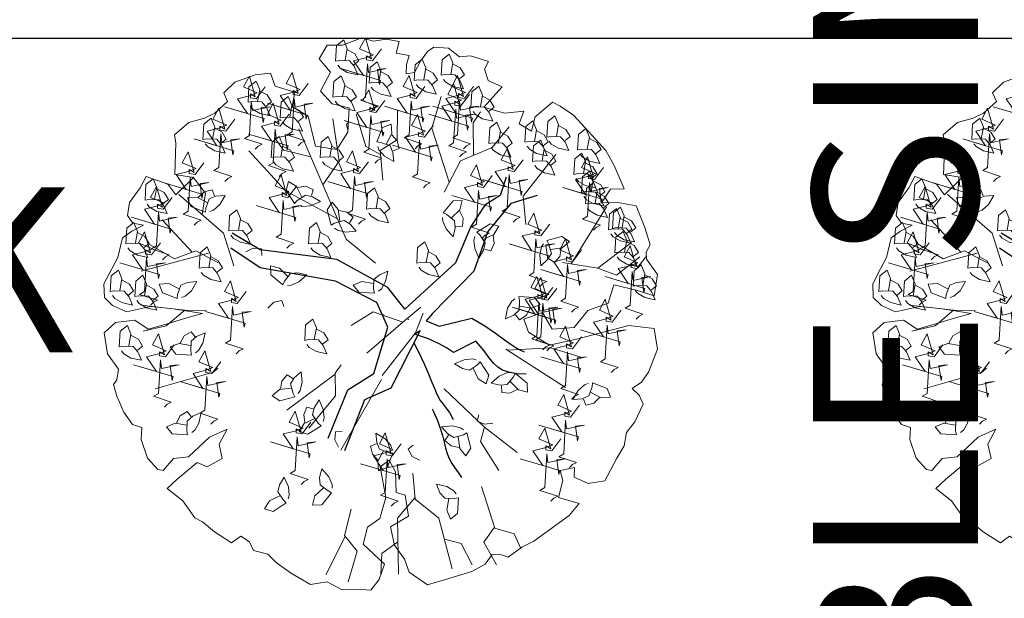
# Model space of a CAD drawing. Units: inches. Extents: x 2831 to 4250, y 1103 to 1797.
# Tile 10 of 15: x 3676 to 3730, y 1690 to 1722. Entities that reach past the tile are written whole.
import ezdxf

# ---------------------------------------------------------------- set-up
doc = ezdxf.new("R2010")
doc.units = ezdxf.units.IN
for name, color, linetype, lineweight in [('A-ANNO-DIMS', 2, 'Continuous', 18), ('A-ANNO-TEXT', 7, 'Continuous', 18), ('A-WALL-PATT', 252, 'Continuous', 13), ('ARBOL', 30, 'Continuous', 13), ('C-PROP', 7, 'Continuous', 25)]:
    doc.layers.add(name, color=color, linetype=linetype, lineweight=lineweight)
doc.layers.add('TALLO', color=36, linetype='Continuous')
doc.styles.get("Standard").update_dxf_attribs({"font": 'arial.ttf'})
doc.dimstyles.new('ISO-25', dxfattribs={"dimtxt": 9, "dimasz": 2.5, "dimexe": 1.25, "dimexo": 0.625, "dimtad": 1, "dimdec": 1, "dimlunit": 3, "dimtxsty": 'Standard', "dimcen": 2.5, "dimadec": 0, "dimazin": 0, "dimtfac": 1, "dimtdec": 1, "dimtmove": 0, "dimatfit": 3, "dimfxl": 1, "dimarcsym": 0})

# ---------------------------------------------------------------- blocks, each defined once
blk = doc.blocks.new('fresno')
at = {"layer": 'ARBOL'}
for p, q in [((2.96, 0.991), (3.575, 1.984)), ((-3.638, 1.194), (-4.164, 1.76)), ((-1.151, -0.932), (-1.99, -1.556)), ((-0.974, -3.757), (-1.31, -4.423))]:
    blk.add_line(p, q, dxfattribs=at)
blk.add_lwpolyline([(0.823, 4.745), (0.566, 4.764), (0.459, 4.687), (0.336, 4.518), (0.233, 4.322), (0.087, 4.298), (0.091, 4.464), (0.14, 4.621), (-0.09, 4.659), (-0.033, 4.863), (-0.264, 4.901), (-0.483, 4.866), (-0.686, 4.924), (-1.021, 4.801), (-1.288, 4.8), (-1.431, 4.563), (-1.234, 4.327), (-1.406, 4), (-1.205, 3.778), (-0.909, 3.705), (-0.931, 3.283), (-1.122, 2.983), (-1.491, 3.043), (-1.619, 3.562), (-1.9, 3.727), (-1.851, 3.982), (-2.197, 4.084), (-2.278, 4.31), (-2.543, 4.283), (-2.896, 4.152), (-3.091, 3.971), (-3.022, 3.817), (-3.244, 3.617), (-3.424, 3.528), (-3.697, 3.455), (-3.946, 3.236), (-3.922, 3.09), (-3.94, 2.548), (-3.617, 2.495), (-3.927, 2.19), (-4.062, 2.379), (-4.443, 2.512), (-4.546, 2.316), (-4.73, 2.062), (-4.767, 1.832), (-4.671, 1.698), (-4.486, 1.667), (-4.693, 1.559), (-4.854, 1.444), (-4.934, 1.102), (-5.037, 0.905), (-5.175, 0.644), (-5.166, 0.406), (-5.024, 0.264), (-4.781, 0.153), (-4.363, 0.249), (-4.014, 0.215), (-3.783, 0.177), (-3.46, 0.124), (-3.733, 0.051), (-4.132, -0.073), (-4.404, -0.146), (-4.639, 0.011), (-4.977, -0.028), (-5.172, -0.209), (-5.113, -0.574), (-4.921, -0.843), (-4.951, -1.027), (-5.012, -1.112), (-4.95, -1.311), (-4.83, -1.592), (-4.676, -1.807), (-4.518, -1.856), (-4.529, -2.068), (-4.417, -2.394), (-4.236, -2.59), (-4.143, -2.605), (-3.967, -2.397), (-3.703, -2.37), (-3.339, -2.027), (-3.032, -1.889), (-3.169, -2.15), (-3.115, -2.396), (-3.376, -2.542), (-3.552, -2.466), (-3.909, -2.762), (-4.077, -2.924), (-3.804, -3.135), (-3.592, -3.43), (-3.461, -3.499), (-3.253, -3.676), (-2.953, -3.867), (-2.792, -3.752), (-2.642, -3.848), (-2.572, -4.001), (-2.323, -4.066), (-2.18, -4.208), (-1.926, -4.392), (-1.58, -4.591), (-1.288, -4.545), (-1.027, -4.683), (-0.788, -4.675), (-0.531, -4.693), (-0.382, -4.505), (-0.29, -4.236), (-0.66, -3.891), (-0.588, -3.595), (-0.374, -3.441), (-0.267, -3.079), (-0.368, -2.541), (-0.208, -2.426), (-0.099, -2.633), (-0.087, -2.991), (0.071, -3.04), (0.129, -3.405), (-0.185, -3.59), (-0.119, -3.909), (0.055, -4.151), (0.136, -4.377), (0.456, -4.596), (0.828, -4.491), (1.227, -4.368), (1.461, -4.241), (1.583, -4.071), (1.748, -4.075), (1.86, -4.117), (2.101, -3.944), (2.308, -3.836), (2.925, -3.393), (3.101, -3.185), (2.74, -3.078), (2.812, -2.782), (2.769, -2.61), (3.015, -2.555), (3.012, -2.721), (3.254, -2.832), (3.546, -2.785), (3.752, -2.393), (3.882, -2.177), (3.92, -1.947), (4.069, -1.758), (4.214, -1.451), (4.144, -1.297), (4.021, -1.182), (4.182, -1.067), (4.304, -0.897), (4.464, -0.497), (4.429, -0.279), (4.406, -0.133), (3.964, -0.083), (3.074, -0.315), (2.582, -0.424), (2.217, -0.197), (2.136, 0.029), (2.462, 0.141), (2.628, -0.147), (3.012, -0.116), (3.249, 0.177), (3.602, 0.308), (3.701, 0.623), (4.089, 0.535), (4.404, 0.436), (4.464, 0.805), (4.272, 1.074), (4.267, 1.193), (4.336, 1.324), (4.243, 1.623), (4.092, 2.003), (3.769, 2.057), (3.485, 2.056), (3.642, 2.291), (3.88, 2.299), (3.71, 2.706), (3.563, 2.967), (3.201, 3.358), (3.001, 3.581), (2.766, 3.738), (2.635, 3.807), (2.332, 3.549), (2.268, 3.299), (2.052, 3.429), (2.136, 3.652), (1.798, 3.613), (1.437, 3.72), (1.755, 4.071), (1.513, 4.182), (1.451, 4.381), (1.519, 4.512), (1.204, 4.611), (1.012, 4.596)], close=True, dxfattribs=at)
for points in [[(-1.104, 4.45), (-1.063, 4.399), (-0.939, 4.325), (-0.757, 4.285), (-0.82, 4.431), (-0.903, 4.527), (-1.075, 4.533), (-1.143, 4.521), (-1.126, 4.792), (-1.002, 4.891), (-0.939, 4.738), (-0.975, 4.535)], [(-0.346, 4.735), (-0.501, 4.528), (-0.605, 4.545), (-0.605, 4.614), (-0.519, 4.563), (-0.622, 4.925), (-0.726, 4.735), (-0.484, 4.632), (-0.622, 4.58), (-0.829, 4.528), (-0.657, 4.27), (-1.053, 4.39), (-0.363, 4.183), (-0.381, 4.114), (-0.415, 4.373), (-0.26, 4.39), (-0.57, 4.321), (-0.588, 4.476), (-0.622, 3.89), (-0.708, 3.839), (-0.398, 3.735), (-0.467, 3.701), (-0.519, 3.649)], [(-0.935, 4.717), (-0.809, 4.65), (-0.736, 4.529), (-0.824, 4.459)], [(0.734, 4.203), (0.775, 4.152), (0.9, 4.078), (1.082, 4.038), (1.018, 4.185), (0.936, 4.281), (0.763, 4.287), (0.696, 4.274), (0.712, 4.546), (0.837, 4.645), (0.899, 4.491), (0.863, 4.289)], [(-0.521, 4.069), (-0.48, 4.018), (-0.356, 3.944), (-0.174, 3.904), (-0.237, 4.051), (-0.32, 4.146), (-0.492, 4.152), (-0.56, 4.14), (-0.543, 4.411), (-0.419, 4.511), (-0.356, 4.357), (-0.392, 4.154)], [(0.263, 4.114), (0.304, 4.063), (0.429, 3.989), (0.611, 3.948), (0.547, 4.095), (0.465, 4.191), (0.293, 4.197), (0.225, 4.185), (0.242, 4.456), (0.366, 4.555), (0.428, 4.402), (0.393, 4.199)], [(0.904, 4.471), (1.029, 4.404), (1.102, 4.282), (1.015, 4.212)], [(-1.623, 4.132), (-1.778, 3.925), (-1.882, 3.942), (-1.882, 4.011), (-1.795, 3.959), (-1.899, 4.321), (-2.002, 4.132), (-1.761, 4.028), (-1.899, 3.977), (-2.106, 3.925), (-1.933, 3.666), (-2.33, 3.787), (-1.64, 3.58), (-1.657, 3.511), (-1.692, 3.77), (-1.537, 3.787), (-1.847, 3.718), (-1.864, 3.873), (-1.899, 3.287), (-1.985, 3.235), (-1.675, 3.132), (-1.744, 3.097), (-1.795, 3.046)], [(-0.352, 4.337), (-0.226, 4.269), (-0.153, 4.148), (-0.241, 4.078)], [(0.433, 4.381), (0.558, 4.314), (0.631, 4.193), (0.544, 4.122)], [(-2.368, 4.073), (-2.523, 3.866), (-2.627, 3.883), (-2.627, 3.952), (-2.541, 3.9), (-2.644, 4.262), (-2.748, 4.073), (-2.506, 3.969), (-2.644, 3.918), (-2.851, 3.866), (-2.679, 3.607), (-3.075, 3.728), (-2.385, 3.521), (-2.403, 3.452), (-2.437, 3.711), (-2.282, 3.728), (-2.592, 3.659), (-2.61, 3.814), (-2.644, 3.228), (-2.73, 3.176), (-2.42, 3.073), (-2.489, 3.038), (-2.541, 2.987)], [(-2.629, 3.733), (-2.588, 3.682), (-2.463, 3.608), (-2.281, 3.568), (-2.345, 3.715), (-2.427, 3.81), (-2.6, 3.816), (-2.667, 3.804), (-2.651, 4.075), (-2.526, 4.175), (-2.464, 4.021), (-2.5, 3.818)], [(-1.149, 3.822), (-1.108, 3.771), (-0.983, 3.697), (-0.802, 3.657), (-0.865, 3.804), (-0.948, 3.9), (-1.12, 3.906), (-1.188, 3.893), (-1.171, 4.165), (-1.047, 4.264), (-0.984, 4.111), (-1.02, 3.908)], [(0.413, 4.08), (0.258, 3.873), (0.154, 3.89), (0.154, 3.959), (0.241, 3.908), (0.137, 4.27), (0.034, 4.08), (0.275, 3.977), (0.137, 3.925), (-0.07, 3.873), (0.103, 3.614), (-0.294, 3.735), (0.396, 3.528), (0.379, 3.459), (0.344, 3.718), (0.499, 3.735), (0.189, 3.666), (0.172, 3.821), (0.137, 3.235), (0.051, 3.183), (0.361, 3.08), (0.292, 3.046), (0.241, 2.994)], [(1.189, 3.942), (1.034, 3.735), (0.931, 3.752), (0.931, 3.821), (1.017, 3.77), (0.913, 4.132), (0.81, 3.942), (1.051, 3.839), (0.913, 3.787), (0.706, 3.735), (0.879, 3.477), (0.482, 3.597), (1.172, 3.39), (1.155, 3.321), (1.12, 3.58), (1.276, 3.597), (0.965, 3.528), (0.948, 3.683), (0.913, 3.097), (0.827, 3.046), (1.138, 2.942), (1.069, 2.908), (1.017, 2.856)], [(1.259, 4.08), (1.103, 3.873), (1, 3.89), (1, 3.959), (1.086, 3.908), (0.982, 4.27), (0.879, 4.08), (1.12, 3.977), (0.982, 3.925), (0.775, 3.873), (0.948, 3.614), (0.551, 3.735), (1.241, 3.528), (1.224, 3.459), (1.189, 3.718), (1.345, 3.735), (1.034, 3.666), (1.017, 3.821), (0.982, 3.235), (0.896, 3.183), (1.207, 3.08), (1.138, 3.046), (1.086, 2.994)], [(-2.459, 4), (-2.334, 3.933), (-2.261, 3.812), (-2.348, 3.742)], [(-0.287, 3.833), (-0.442, 3.626), (-0.546, 3.643), (-0.546, 3.712), (-0.46, 3.661), (-0.563, 4.023), (-0.667, 3.833), (-0.425, 3.73), (-0.563, 3.678), (-0.77, 3.626), (-0.598, 3.367), (-0.995, 3.488), (-0.304, 3.281), (-0.322, 3.212), (-0.356, 3.471), (-0.201, 3.488), (-0.511, 3.419), (-0.529, 3.574), (-0.563, 2.988), (-0.649, 2.936), (-0.339, 2.833), (-0.408, 2.799), (-0.46, 2.747)], [(-0.98, 4.09), (-0.854, 4.023), (-0.781, 3.901), (-0.869, 3.831)], [(1.25, 3.643), (1.291, 3.592), (1.416, 3.518), (1.597, 3.478), (1.534, 3.625), (1.451, 3.721), (1.279, 3.727), (1.211, 3.714), (1.228, 3.985), (1.352, 4.085), (1.415, 3.931), (1.379, 3.729)], [(-1.951, 3.597), (-2.106, 3.39), (-2.209, 3.408), (-2.209, 3.477), (-2.123, 3.425), (-2.227, 3.787), (-2.33, 3.597), (-2.089, 3.494), (-2.227, 3.442), (-2.434, 3.39), (-2.261, 3.132), (-2.658, 3.252), (-1.968, 3.046), (-1.985, 2.977), (-2.02, 3.235), (-1.864, 3.252), (-2.175, 3.183), (-2.192, 3.339), (-2.227, 2.752), (-2.313, 2.701), (-2.002, 2.597), (-2.071, 2.563), (-2.123, 2.511)], [(-2.068, 3.464), (-2.027, 3.413), (-1.903, 3.339), (-1.721, 3.299), (-1.784, 3.446), (-1.867, 3.542), (-2.039, 3.547), (-2.107, 3.535), (-2.09, 3.806), (-1.966, 3.906), (-1.903, 3.752), (-1.939, 3.55)], [(0.837, 2.414), (0.533, 3.352), (0.697, 3.906)], [(1.419, 3.911), (1.545, 3.844), (1.618, 3.722), (1.53, 3.652)], [(-2.898, 3.511), (-3.053, 3.304), (-3.157, 3.321), (-3.157, 3.39), (-3.071, 3.339), (-3.174, 3.701), (-3.278, 3.511), (-3.036, 3.408), (-3.174, 3.356), (-3.381, 3.304), (-3.209, 3.046), (-3.605, 3.166), (-2.915, 2.959), (-2.932, 2.89), (-2.967, 3.149), (-2.812, 3.166), (-3.122, 3.097), (-3.14, 3.253), (-3.174, 2.666), (-3.26, 2.615), (-2.95, 2.511), (-3.019, 2.477), (-3.071, 2.425)], [(-1.899, 3.732), (-1.773, 3.664), (-1.7, 3.543), (-1.788, 3.473)], [(-0.063, 3.671), (-0.069, 3.151), (-0.364, 2.965), (-0.319, 2.449)], [(1.259, 2.882), (1.254, 3.446), (1.381, 3.636)], [(-3.413, 3.083), (-3.373, 3.032), (-3.248, 2.958), (-3.066, 2.918), (-3.129, 3.065), (-3.212, 3.161), (-3.384, 3.167), (-3.452, 3.154), (-3.435, 3.425), (-3.311, 3.525), (-3.248, 3.371), (-3.284, 3.169)], [(-1.367, 2.367), (-1.081, 2.78), (-1.193, 3.514)], [(-0.923, 3.449), (-0.951, 3.425), (-0.93, 3.313)], [(-0.358, 2.895), (-0.615, 3.037), (-0.783, 3.596)], [(0.558, 3.402), (0.403, 3.195), (0.299, 3.212), (0.299, 3.281), (0.386, 3.23), (0.282, 3.592), (0.179, 3.402), (0.42, 3.299), (0.282, 3.247), (0.075, 3.195), (0.248, 2.936), (-0.149, 3.057), (0.541, 2.85), (0.524, 2.781), (0.489, 3.04), (0.644, 3.057), (0.334, 2.988), (0.317, 3.143), (0.282, 2.557), (0.196, 2.505), (0.506, 2.402), (0.437, 2.368), (0.386, 2.316)], [(1.564, 3.016), (1.605, 2.965), (1.729, 2.891), (1.911, 2.851), (1.848, 2.998), (1.765, 3.094), (1.593, 3.099), (1.525, 3.087), (1.542, 3.358), (1.666, 3.458), (1.729, 3.304), (1.693, 3.102)], [(2.191, 3.038), (2.232, 2.987), (2.357, 2.913), (2.539, 2.873), (2.475, 3.02), (2.393, 3.116), (2.221, 3.122), (2.153, 3.109), (2.17, 3.381), (2.294, 3.48), (2.356, 3.326), (2.321, 3.124)], [(2.573, 3.128), (2.613, 3.077), (2.738, 3.003), (2.92, 2.963), (2.857, 3.11), (2.774, 3.205), (2.602, 3.211), (2.534, 3.199), (2.551, 3.47), (2.675, 3.57), (2.738, 3.416), (2.702, 3.214)], [(-3.244, 3.351), (-3.118, 3.284), (-3.045, 3.162), (-3.133, 3.092)], [(-0.448, 1), (-0.961, 1.419), (-1.784, 3.341)], [(-0.41, 3.035), (-0.387, 2.974), (-0.291, 2.865), (-0.131, 2.771), (-0.146, 2.93), (-0.195, 3.047), (-0.357, 3.106), (-0.425, 3.115), (-0.325, 3.368), (-0.176, 3.424), (-0.164, 3.258), (-0.261, 3.077)], [(0.746, 2.242), (1.034, 2.786), (1.584, 3.019), (1.879, 3.374)], [(1.733, 3.284), (1.859, 3.216), (1.932, 3.095), (1.844, 3.025)], [(2.361, 3.306), (2.486, 3.239), (2.559, 3.117), (2.472, 3.047)], [(2.742, 3.396), (2.868, 3.328), (2.941, 3.207), (2.853, 3.137)], [(3.111, 2.904), (3.152, 2.853), (3.276, 2.779), (3.458, 2.739), (3.395, 2.886), (3.312, 2.981), (3.14, 2.987), (3.072, 2.975), (3.089, 3.246), (3.213, 3.346), (3.276, 3.192), (3.24, 2.99)], [(-2.225, 2.77), (-2.184, 2.718), (-2.06, 2.645), (-1.878, 2.604), (-1.941, 2.751), (-2.024, 2.847), (-2.196, 2.853), (-2.264, 2.84), (-2.247, 3.112), (-2.123, 3.211), (-2.06, 3.058), (-2.096, 2.855)], [(-1.575, 2.854), (-2.052, 2.969), (-2.2, 3.178)], [(-1.373, 2.77), (-1.332, 2.718), (-1.208, 2.645), (-1.026, 2.604), (-1.089, 2.751), (-1.172, 2.847), (-1.344, 2.853), (-1.412, 2.84), (-1.395, 3.112), (-1.271, 3.211), (-1.208, 3.058), (-1.244, 2.855)], [(-0.166, 3.238), (-0.068, 3.135), (-0.036, 2.997), (-0.141, 2.957)], [(2.326, 2.702), (2.367, 2.651), (2.492, 2.577), (2.673, 2.537), (2.61, 2.684), (2.527, 2.78), (2.355, 2.786), (2.287, 2.773), (2.304, 3.045), (2.428, 3.144), (2.491, 2.99), (2.455, 2.788)], [(3.28, 3.172), (3.406, 3.104), (3.479, 2.983), (3.391, 2.913)], [(-3.434, 2.752), (-3.59, 2.546), (-3.693, 2.563), (-3.693, 2.632), (-3.607, 2.58), (-3.71, 2.942), (-3.814, 2.752), (-3.572, 2.649), (-3.71, 2.597), (-3.917, 2.546), (-3.745, 2.287), (-4.142, 2.408), (-3.452, 2.201), (-3.469, 2.132), (-3.503, 2.39), (-3.348, 2.408), (-3.659, 2.339), (-3.676, 2.494), (-3.71, 1.908), (-3.797, 1.856), (-3.486, 1.753), (-3.555, 1.718), (-3.607, 1.666)], [(-1.112, 1.773), (-2.014, 2.265), (-2.654, 2.957)], [(-2.056, 3.037), (-1.93, 2.97), (-1.857, 2.849), (-1.945, 2.778)], [(-0.57, 2.77), (-0.726, 2.563), (-0.829, 2.58), (-0.829, 2.649), (-0.743, 2.597), (-0.846, 2.959), (-0.95, 2.77), (-0.708, 2.666), (-0.846, 2.615), (-1.053, 2.563), (-0.881, 2.304), (-1.278, 2.425), (-0.588, 2.218), (-0.605, 2.149), (-0.639, 2.408), (-0.484, 2.425), (-0.795, 2.356), (-0.812, 2.511), (-0.846, 1.925), (-0.933, 1.873), (-0.622, 1.77), (-0.691, 1.735), (-0.743, 1.684)], [(-1.204, 3.037), (-1.078, 2.97), (-1.005, 2.849), (-1.093, 2.778)], [(2.121, 2.804), (1.966, 2.597), (1.862, 2.615), (1.862, 2.683), (1.949, 2.632), (1.845, 2.994), (1.742, 2.804), (1.983, 2.701), (1.845, 2.649), (1.638, 2.597), (1.811, 2.339), (1.414, 2.459), (2.104, 2.252), (2.087, 2.184), (2.052, 2.442), (2.207, 2.459), (1.897, 2.39), (1.88, 2.546), (1.845, 1.959), (1.759, 1.908), (2.069, 1.804), (2, 1.77), (1.949, 1.718)], [(2.495, 2.97), (2.621, 2.903), (2.694, 2.781), (2.606, 2.711)], [(3.043, 2.478), (3.084, 2.427), (3.209, 2.353), (3.391, 2.313), (3.327, 2.46), (3.245, 2.556), (3.073, 2.562), (3.005, 2.549), (3.022, 2.82), (3.146, 2.92), (3.208, 2.766), (3.173, 2.564)], [(2.171, 1.674), (2.121, 2.172), (2.689, 2.898)], [(3.519, 2.666), (3.363, 2.459), (3.26, 2.477), (3.26, 2.546), (3.346, 2.494), (3.243, 2.856), (3.139, 2.666), (3.381, 2.563), (3.243, 2.511), (3.036, 2.459), (3.208, 2.201), (2.811, 2.321), (3.501, 2.115), (3.484, 2.046), (3.45, 2.304), (3.605, 2.321), (3.294, 2.252), (3.277, 2.408), (3.243, 1.821), (3.156, 1.77), (3.467, 1.666), (3.398, 1.632), (3.346, 1.58)], [(3.213, 2.746), (3.338, 2.679), (3.411, 2.557), (3.324, 2.487)], [(1.586, 2.528), (1.431, 2.321), (1.327, 2.339), (1.327, 2.408), (1.414, 2.356), (1.31, 2.718), (1.207, 2.528), (1.448, 2.425), (1.31, 2.373), (1.103, 2.321), (1.276, 2.063), (0.879, 2.184), (1.569, 1.977), (1.552, 1.908), (1.517, 2.166), (1.673, 2.184), (1.362, 2.115), (1.345, 2.27), (1.31, 1.684), (1.224, 1.632), (1.535, 1.528), (1.466, 1.494), (1.414, 1.442)], [(3.178, 2.165), (3.219, 2.113), (3.344, 2.04), (3.525, 1.999), (3.462, 2.146), (3.379, 2.242), (3.207, 2.248), (3.139, 2.236), (3.156, 2.507), (3.28, 2.606), (3.343, 2.453), (3.307, 2.25)], [(-4.422, 2.03), (-4.381, 1.979), (-4.257, 1.905), (-4.075, 1.865), (-4.138, 2.012), (-4.221, 2.108), (-4.393, 2.114), (-4.461, 2.101), (-4.444, 2.372), (-4.32, 2.472), (-4.257, 2.318), (-4.293, 2.116)], [(-3.468, 1.85), (-3.409, 2.222), (-3.628, 2.505)], [(-1.817, 2.351), (-1.972, 2.144), (-2.075, 2.162), (-2.075, 2.231), (-1.989, 2.179), (-2.093, 2.541), (-2.196, 2.351), (-1.955, 2.248), (-2.093, 2.196), (-2.3, 2.144), (-2.127, 1.886), (-2.524, 2.006), (-1.834, 1.8), (-1.851, 1.731), (-1.886, 1.989), (-1.73, 2.006), (-2.041, 1.937), (-2.058, 2.093), (-2.093, 1.506), (-2.179, 1.455), (-1.868, 1.351), (-1.937, 1.317), (-1.989, 1.265)], [(-1.786, 2.007), (-1.722, 1.99), (-1.578, 2.003), (-1.407, 2.078), (-1.545, 2.159), (-1.668, 2.188), (-1.811, 2.092), (-1.859, 2.042), (-2.004, 2.271), (-1.962, 2.425), (-1.821, 2.337), (-1.731, 2.152)], [(3.245, 1.963), (3.286, 1.912), (3.411, 1.838), (3.593, 1.798), (3.529, 1.945), (3.447, 2.041), (3.274, 2.046), (3.206, 2.034), (3.223, 2.305), (3.347, 2.405), (3.41, 2.251), (3.374, 2.049)], [(3.347, 2.432), (3.473, 2.365), (3.546, 2.244), (3.458, 2.173)], [(-3.986, 2.149), (-4.142, 1.942), (-4.245, 1.959), (-4.245, 2.028), (-4.159, 1.977), (-4.262, 2.339), (-4.366, 2.149), (-4.124, 2.046), (-4.262, 1.994), (-4.47, 1.942), (-4.297, 1.684), (-4.694, 1.804), (-4.004, 1.597), (-4.021, 1.528), (-4.055, 1.787), (-3.9, 1.804), (-4.211, 1.735), (-4.228, 1.89), (-4.262, 1.304), (-4.349, 1.253), (-4.038, 1.149), (-4.107, 1.115), (-4.159, 1.063)], [(-4.253, 2.298), (-4.127, 2.231), (-4.054, 2.109), (-4.142, 2.039)], [(-3.533, 2.149), (-3.43, 2.247), (-3.292, 2.279), (-3.252, 2.174)], [(-1.806, 2.323), (-1.665, 2.343), (-1.534, 2.287), (-1.564, 2.179)], [(-0.566, 1.873), (-0.525, 1.822), (-0.4, 1.748), (-0.219, 1.708), (-0.282, 1.855), (-0.365, 1.951), (-0.537, 1.957), (-0.605, 1.944), (-0.588, 2.216), (-0.464, 2.315), (-0.401, 2.162), (-0.437, 1.959)], [(3.415, 2.231), (3.54, 2.163), (3.613, 2.042), (3.525, 1.972)], [(-2.916, 0.958), (-3.096, 1.528), (-3.871, 2.197)], [(-3.331, 1.905), (-3.269, 1.928), (-3.161, 2.024), (-3.066, 2.184), (-3.226, 2.169), (-3.342, 2.121), (-3.401, 1.958), (-3.41, 1.89), (-3.663, 1.99), (-3.719, 2.139), (-3.554, 2.151), (-3.372, 2.054)], [(-1.164, 1.612), (-1.109, 1.576), (-0.967, 1.544), (-0.782, 1.562), (-0.888, 1.682), (-0.996, 1.748), (-1.162, 1.7), (-1.222, 1.667), (-1.29, 1.93), (-1.203, 2.063), (-1.096, 1.937), (-1.067, 1.733)], [(-0.397, 2.141), (-0.271, 2.074), (-0.198, 1.952), (-0.286, 1.882)], [(0.72, 1.798), (0.723, 1.733), (0.781, 1.6), (0.904, 1.46), (0.939, 1.616), (0.929, 1.742), (0.793, 1.848), (0.73, 1.878), (0.904, 2.088), (1.062, 2.095), (1.023, 1.934), (0.875, 1.791)], [(-2.965, 1.493), (-2.924, 1.441), (-2.799, 1.368), (-2.618, 1.327), (-2.681, 1.474), (-2.764, 1.57), (-2.936, 1.576), (-3.004, 1.564), (-2.987, 1.835), (-2.863, 1.934), (-2.8, 1.781), (-2.836, 1.578)], [(-1.085, 1.919), (-0.945, 1.893), (-0.838, 1.801), (-0.9, 1.707)], [(1.014, 1.915), (1.077, 1.787), (1.064, 1.646), (0.952, 1.64)], [(3.649, 1.515), (3.69, 1.464), (3.814, 1.39), (3.996, 1.35), (3.933, 1.497), (3.85, 1.592), (3.678, 1.598), (3.61, 1.586), (3.627, 1.857), (3.751, 1.957), (3.814, 1.803), (3.778, 1.601)], [(3.716, 1.537), (3.757, 1.486), (3.882, 1.412), (4.063, 1.372), (4, 1.519), (3.917, 1.615), (3.745, 1.621), (3.677, 1.608), (3.694, 1.88), (3.818, 1.979), (3.881, 1.825), (3.845, 1.623)], [(-2.796, 1.76), (-2.67, 1.693), (-2.597, 1.572), (-2.685, 1.501)], [(2.587, 1.684), (2.432, 1.477), (2.328, 1.494), (2.328, 1.563), (2.414, 1.511), (2.311, 1.873), (2.207, 1.684), (2.449, 1.58), (2.311, 1.528), (2.104, 1.477), (2.276, 1.218), (1.88, 1.339), (2.57, 1.132), (2.552, 1.063), (2.518, 1.321), (2.673, 1.339), (2.363, 1.27), (2.345, 1.425), (2.311, 0.839), (2.225, 0.787), (2.535, 0.684), (2.466, 0.649), (2.414, 0.597)], [(3.818, 1.783), (3.944, 1.715), (4.017, 1.594), (3.929, 1.524)], [(3.885, 1.805), (4.011, 1.738), (4.084, 1.616), (3.996, 1.546)], [(-4.193, 1.356), (-4.349, 1.149), (-4.452, 1.166), (-4.452, 1.235), (-4.366, 1.184), (-4.469, 1.546), (-4.573, 1.356), (-4.331, 1.253), (-4.469, 1.201), (-4.677, 1.149), (-4.504, 0.89), (-4.901, 1.011), (-4.211, 0.804), (-4.228, 0.735), (-4.262, 0.994), (-4.107, 1.011), (-4.418, 0.942), (-4.435, 1.097), (-4.469, 0.511), (-4.556, 0.459), (-4.245, 0.356), (-4.314, 0.322), (-4.366, 0.27)], [(-4.759, 1.269), (-4.718, 1.217), (-4.593, 1.144), (-4.411, 1.103), (-4.475, 1.25), (-4.557, 1.346), (-4.729, 1.352), (-4.797, 1.339), (-4.78, 1.611), (-4.656, 1.71), (-4.594, 1.557), (-4.629, 1.354)], [(-1.575, 1.269), (-1.534, 1.217), (-1.409, 1.144), (-1.228, 1.103), (-1.291, 1.25), (-1.373, 1.346), (-1.546, 1.352), (-1.614, 1.339), (-1.597, 1.611), (-1.473, 1.71), (-1.41, 1.557), (-1.446, 1.354)], [(1.283, 1.469), (1.266, 1.405), (1.279, 1.261), (1.354, 1.09), (1.435, 1.228), (1.464, 1.351), (1.368, 1.494), (1.318, 1.542), (1.547, 1.687), (1.7, 1.645), (1.613, 1.504), (1.428, 1.414)], [(3.761, 1.112), (3.802, 1.061), (3.926, 0.987), (4.108, 0.947), (4.045, 1.093), (3.962, 1.189), (3.79, 1.195), (3.722, 1.183), (3.739, 1.454), (3.863, 1.553), (3.926, 1.4), (3.89, 1.197)], [(-4.589, 1.536), (-4.464, 1.469), (-4.391, 1.348), (-4.478, 1.277)], [(-1.406, 1.536), (-1.28, 1.469), (-1.207, 1.348), (-1.295, 1.277)], [(0.308, 0.933), (0.349, 0.881), (0.474, 0.807), (0.656, 0.767), (0.592, 0.914), (0.51, 1.01), (0.337, 1.016), (0.27, 1.003), (0.286, 1.275), (0.411, 1.374), (0.473, 1.221), (0.437, 1.018)], [(1.599, 1.489), (1.618, 1.348), (1.563, 1.217), (1.455, 1.247)], [(2.479, 1.34), (2.443, 1.285), (2.411, 1.143), (2.429, 0.958), (2.549, 1.064), (2.615, 1.172), (2.567, 1.338), (2.534, 1.398), (2.797, 1.466), (2.93, 1.379), (2.804, 1.272), (2.6, 1.243)], [(3.139, 1.235), (2.984, 1.028), (2.88, 1.046), (2.88, 1.115), (2.967, 1.063), (2.863, 1.425), (2.759, 1.235), (3.001, 1.132), (2.863, 1.08), (2.656, 1.028), (2.828, 0.77), (2.432, 0.891), (3.122, 0.684), (3.105, 0.615), (3.07, 0.873), (3.225, 0.891), (2.915, 0.822), (2.897, 0.977), (2.863, 0.391), (2.777, 0.339), (3.087, 0.235), (3.018, 0.201), (2.967, 0.149)], [(3.93, 1.379), (4.056, 1.312), (4.129, 1.191), (4.041, 1.121)], [(-3.192, 1.017), (-3.578, 1.215), (-3.949, 1.081), (-4.398, 1.339)], [(-3.481, 0.843), (-3.44, 0.792), (-3.315, 0.718), (-3.133, 0.678), (-3.197, 0.825), (-3.279, 0.92), (-3.451, 0.926), (-3.519, 0.914), (-3.502, 1.185), (-3.378, 1.285), (-3.316, 1.131), (-3.351, 0.928)], [(-2.703, 1.201), (-2.575, 1.263), (-2.433, 1.251), (-2.428, 1.139)], [(0.478, 1.2), (0.603, 1.133), (0.676, 1.011), (0.589, 0.941)], [(2.786, 1.261), (2.76, 1.121), (2.668, 1.014), (2.574, 1.076)], [(4.01, 1.36), (3.422, 0.918)], [(4.26, 1.115), (4.105, 0.908), (4.002, 0.925), (4.002, 0.994), (4.088, 0.942), (3.984, 1.304), (3.881, 1.115), (4.122, 1.011), (3.984, 0.959), (3.777, 0.908), (3.95, 0.649), (3.553, 0.77), (4.243, 0.563), (4.226, 0.494), (4.191, 0.753), (4.347, 0.77), (4.036, 0.701), (4.019, 0.856), (3.984, 0.27), (3.898, 0.218), (4.209, 0.115), (4.14, 0.08), (4.088, 0.029)], [(-3.354, 1.176), (-4.529, 0.864)], [(-3.311, 1.111), (-3.186, 1.043), (-3.113, 0.922), (-3.2, 0.852)], [(2.808, 1.015), (3.422, 0.918), (3.422, 0.918), (3.748, 0.794), (4.154, 1.111)], [(-5.028, 0.44), (-4.987, 0.388), (-4.862, 0.315), (-4.68, 0.274), (-4.744, 0.421), (-4.826, 0.517), (-4.998, 0.523), (-5.066, 0.511), (-5.049, 0.782), (-4.925, 0.881), (-4.863, 0.728), (-4.898, 0.525)], [(-1.981, 0.615), (-1.915, 0.618), (-1.782, 0.676), (-1.643, 0.799), (-1.799, 0.834), (-1.925, 0.824), (-2.031, 0.688), (-2.061, 0.626), (-2.27, 0.799), (-2.278, 0.958), (-2.117, 0.918), (-1.974, 0.77)], [(-0.397, 0.517), (-0.346, 0.557), (-0.272, 0.682), (-0.232, 0.864), (-0.379, 0.801), (-0.474, 0.718), (-0.48, 0.546), (-0.468, 0.478), (-0.739, 0.495), (-0.838, 0.619), (-0.685, 0.682), (-0.482, 0.646)], [(4.075, 0.529), (4.116, 0.478), (4.24, 0.404), (4.422, 0.364), (4.359, 0.511), (4.276, 0.607), (4.104, 0.613), (4.036, 0.6), (4.053, 0.871), (4.177, 0.971), (4.24, 0.817), (4.204, 0.615)], [(-4.858, 0.707), (-4.733, 0.64), (-4.66, 0.519), (-4.747, 0.448)], [(-4.602, 0.35), (-4.561, 0.299), (-4.436, 0.225), (-4.254, 0.185), (-4.318, 0.332), (-4.4, 0.428), (-4.572, 0.433), (-4.64, 0.421), (-4.623, 0.692), (-4.499, 0.792), (-4.437, 0.638), (-4.472, 0.436)], [(-2.698, 0.509), (-2.854, 0.302), (-2.957, 0.319), (-2.957, 0.388), (-2.871, 0.336), (-2.974, 0.698), (-3.078, 0.509), (-2.836, 0.405), (-2.974, 0.353), (-3.182, 0.302), (-3.009, 0.043), (-3.406, 0.164), (-2.716, -0.043), (-2.733, -0.112), (-2.767, 0.147), (-2.612, 0.164), (-2.923, 0.095), (-2.94, 0.25), (-2.974, -0.336), (-3.061, -0.388), (-2.75, -0.491), (-2.819, -0.526), (-2.871, -0.577)], [(2.639, 0.58), (2.483, 0.373), (2.38, 0.391), (2.38, 0.46), (2.466, 0.408), (2.363, 0.77), (2.259, 0.58), (2.501, 0.477), (2.363, 0.425), (2.156, 0.373), (2.328, 0.115), (1.931, 0.235), (2.621, 0.029), (2.604, -0.04), (2.57, 0.218), (2.725, 0.235), (2.414, 0.166), (2.397, 0.322), (2.363, -0.265), (2.276, -0.316), (2.587, -0.42), (2.518, -0.454), (2.466, -0.506)], [(2.708, 0.563), (2.552, 0.356), (2.449, 0.373), (2.449, 0.442), (2.535, 0.391), (2.432, 0.753), (2.328, 0.563), (2.57, 0.46), (2.432, 0.408), (2.225, 0.356), (2.397, 0.097), (2, 0.218), (2.69, 0.011), (2.673, -0.058), (2.639, 0.201), (2.794, 0.218), (2.483, 0.149), (2.466, 0.304), (2.432, -0.282), (2.345, -0.334), (2.656, -0.437), (2.587, -0.471), (2.535, -0.523)], [(4.244, 0.797), (4.37, 0.73), (4.443, 0.608), (4.355, 0.538)], [(-4.432, 0.618), (-4.307, 0.55), (-4.234, 0.429), (-4.321, 0.359)], [(-3.824, 0.404), (-3.763, 0.427), (-3.654, 0.523), (-3.559, 0.683), (-3.719, 0.668), (-3.835, 0.62), (-3.894, 0.457), (-3.903, 0.389), (-4.156, 0.489), (-4.212, 0.638), (-4.047, 0.65), (-3.865, 0.553)], [(-2.322, 0.222), (-2.219, 0.321), (-2.081, 0.353), (-2.042, 0.248)], [(1.978, 0.384), (1.927, 0.343), (1.853, 0.218), (1.813, 0.036), (1.96, 0.1), (2.056, 0.182), (2.061, 0.355), (2.049, 0.422), (2.32, 0.406), (2.42, 0.281), (2.266, 0.219), (2.064, 0.254)], [(3.829, 0.184), (3.674, -0.023), (3.57, -0.006), (3.57, 0.063), (3.657, 0.011), (3.553, 0.373), (3.45, 0.184), (3.691, 0.08), (3.553, 0.029), (3.346, -0.023), (3.519, -0.282), (3.122, -0.161), (3.812, -0.368), (3.795, -0.437), (3.76, -0.178), (3.915, -0.161), (3.605, -0.23), (3.588, -0.075), (3.553, -0.661), (3.467, -0.713), (3.777, -0.816), (3.708, -0.851), (3.657, -0.902)], [(-3.394, 0.18), (-3.77, 0.182), (-4.532, 0.27)], [(-3.77, 0.182), (-4.09, -0.088), (-4.494, -0.18)], [(-0.596, -0.564), (0.03, -0.026), (0.339, 0.235)], [(2.246, 0.214), (2.178, 0.089), (2.057, 0.016), (1.987, 0.103)], [(-1.642, -0.412), (-1.601, -0.463), (-1.477, -0.537), (-1.295, -0.577), (-1.358, -0.43), (-1.441, -0.334), (-1.613, -0.328), (-1.681, -0.341), (-1.664, -0.069), (-1.54, 0.03), (-1.477, -0.124), (-1.513, -0.326)], [(0.03, -0.026), (-0.491, 0.154), (-0.871, -0.08)], [(0.38, 0.131), (0.248, -0.21), (-0.33, -0.951)], [(-4.871, -0.524), (-4.83, -0.575), (-4.705, -0.649), (-4.523, -0.689), (-4.587, -0.542), (-4.669, -0.446), (-4.841, -0.44), (-4.909, -0.453), (-4.893, -0.181), (-4.768, -0.082), (-4.706, -0.236), (-4.741, -0.438)], [(-1.473, -0.144), (-1.347, -0.211), (-1.274, -0.333), (-1.362, -0.403)], [(3.139, -0.282), (2.984, -0.489), (2.88, -0.471), (2.88, -0.402), (2.967, -0.454), (2.863, -0.092), (2.759, -0.282), (3.001, -0.385), (2.863, -0.437), (2.656, -0.489), (2.828, -0.747), (2.432, -0.627), (3.122, -0.834), (3.105, -0.902), (3.07, -0.644), (3.225, -0.627), (2.915, -0.696), (2.897, -0.54), (2.863, -1.127), (2.777, -1.178), (3.087, -1.282), (3.018, -1.316), (2.967, -1.368)], [(-4.701, -0.256), (-4.576, -0.323), (-4.503, -0.445), (-4.59, -0.515)], [(-3.952, -0.42), (-4.107, -0.627), (-4.211, -0.609), (-4.211, -0.54), (-4.124, -0.592), (-4.228, -0.23), (-4.331, -0.42), (-4.09, -0.523), (-4.228, -0.575), (-4.435, -0.627), (-4.262, -0.885), (-4.659, -0.765), (-3.969, -0.971), (-3.986, -1.04), (-4.021, -0.782), (-3.866, -0.765), (-4.176, -0.834), (-4.193, -0.678), (-4.228, -1.265), (-4.314, -1.316), (-4.004, -1.42), (-4.073, -1.454), (-4.124, -1.506)], [(-3.58, -0.559), (-3.529, -0.518), (-3.455, -0.393), (-3.415, -0.211), (-3.562, -0.275), (-3.658, -0.357), (-3.664, -0.53), (-3.651, -0.597), (-3.923, -0.581), (-4.022, -0.456), (-3.868, -0.394), (-3.666, -0.43)], [(-3.848, -0.389), (-3.781, -0.264), (-3.659, -0.191), (-3.589, -0.278)], [(1.822, -0.495), (2.859, -1.165)], [(1.846, -0.51), (2.605, -0.469), (3.129, -0.637)], [(-3.141, -0.713), (-3.296, -0.92), (-3.4, -0.902), (-3.4, -0.834), (-3.314, -0.885), (-3.417, -0.523), (-3.521, -0.713), (-3.279, -0.816), (-3.417, -0.868), (-3.624, -0.92), (-3.452, -1.178), (-3.848, -1.058), (-3.158, -1.265), (-3.175, -1.333), (-3.21, -1.075), (-3.055, -1.058), (-3.365, -1.127), (-3.383, -0.971), (-3.417, -1.558), (-3.503, -1.609), (-3.193, -1.713), (-3.262, -1.747), (-3.314, -1.799)], [(1.304, -0.681), (1.241, -0.664), (1.097, -0.678), (0.926, -0.752), (1.064, -0.833), (1.187, -0.862), (1.33, -0.766), (1.377, -0.716), (1.523, -0.945), (1.481, -1.099), (1.34, -1.011), (1.25, -0.826)], [(-3.195, -0.824), (-3.267, -0.898), (-4.285, -1.185)], [(-1.047, -0.767), (-1.151, -0.913), (-1.144, -1.307), (-1.61, -1.871)], [(-1.794, -1.268), (-1.758, -1.214), (-1.726, -1.072), (-1.744, -0.887), (-1.865, -0.993), (-1.93, -1.101), (-1.883, -1.266), (-1.85, -1.327), (-2.113, -1.395), (-2.246, -1.307), (-2.119, -1.2), (-1.916, -1.172)], [(-2.101, -1.19), (-2.076, -1.05), (-1.983, -0.943), (-1.889, -1.004)], [(-0.346, -1.024), (-1.05, -2.251)], [(1.903, -0.903), (1.837, -0.905), (1.704, -0.963), (1.565, -1.086), (1.721, -1.122), (1.847, -1.111), (1.953, -0.975), (1.983, -0.913), (2.192, -1.086), (2.2, -1.245), (2.039, -1.205), (1.896, -1.057)], [(0.748, -1.185), (1.452, -1.855), (2.021, -2.292)], [(2.02, -1.197), (1.891, -1.259), (1.75, -1.247), (1.745, -1.134)], [(3.253, -1.094), (3.192, -1.117), (3.083, -1.213), (2.988, -1.374), (3.148, -1.359), (3.264, -1.31), (3.323, -1.148), (3.332, -1.079), (3.585, -1.179), (3.641, -1.328), (3.476, -1.34), (3.294, -1.244)], [(3.105, -1.471), (2.949, -1.678), (2.846, -1.661), (2.846, -1.592), (2.932, -1.644), (2.829, -1.282), (2.725, -1.471), (2.967, -1.575), (2.829, -1.627), (2.621, -1.678), (2.794, -1.937), (2.397, -1.816), (3.087, -2.023), (3.07, -2.092), (3.036, -1.833), (3.191, -1.816), (2.88, -1.885), (2.863, -1.73), (2.829, -2.316), (2.742, -2.368), (3.053, -2.471), (2.984, -2.506), (2.932, -2.558)], [(3.455, -1.338), (3.352, -1.437), (3.214, -1.469), (3.175, -1.364)], [(-1.361, -1.756), (-1.343, -1.693), (-1.357, -1.548), (-1.431, -1.377), (-1.513, -1.515), (-1.542, -1.638), (-1.445, -1.781), (-1.395, -1.829), (-1.625, -1.974), (-1.778, -1.932), (-1.691, -1.791), (-1.506, -1.701)], [(-1.677, -1.776), (-1.696, -1.635), (-1.641, -1.504), (-1.533, -1.534)], [(-3.648, -1.948), (-3.596, -1.907), (-3.523, -1.782), (-3.482, -1.6), (-3.629, -1.664), (-3.725, -1.746), (-3.731, -1.919), (-3.719, -1.986), (-3.99, -1.97), (-4.089, -1.845), (-3.936, -1.783), (-3.733, -1.819)], [(-3.915, -1.778), (-3.848, -1.653), (-3.727, -1.58), (-3.656, -1.667)], [(-1.571, -1.764), (-1.726, -1.971), (-1.83, -1.954), (-1.83, -1.885), (-1.744, -1.937), (-1.847, -1.575), (-1.951, -1.764), (-1.709, -1.868), (-1.847, -1.92), (-2.054, -1.971), (-1.882, -2.23), (-2.278, -2.109), (-1.588, -2.316), (-1.605, -2.385), (-1.64, -2.127), (-1.485, -2.109), (-1.795, -2.178), (-1.813, -2.023), (-1.847, -2.609), (-1.933, -2.661), (-1.623, -2.764), (-1.692, -2.799), (-1.744, -2.851)], [(1.593, -1.781), (1.452, -1.801), (1.322, -1.746), (1.352, -1.637)], [(1.086, -1.899), (1.031, -1.863), (0.89, -1.831), (0.704, -1.849), (0.81, -1.969), (0.918, -2.035), (1.084, -1.987), (1.145, -1.954), (1.212, -2.218), (1.125, -2.35), (1.018, -2.224), (0.989, -2.02)], [(1.452, -1.855), (1.379, -2.105), (1.698, -2.609)], [(2.777, -2.058), (2.621, -2.264), (2.518, -2.247), (2.518, -2.178), (2.604, -2.23), (2.501, -1.868), (2.397, -2.058), (2.639, -2.161), (2.501, -2.213), (2.294, -2.264), (2.466, -2.523), (2.069, -2.402), (2.759, -2.609), (2.742, -2.678), (2.708, -2.42), (2.863, -2.402), (2.552, -2.471), (2.535, -2.316), (2.501, -2.902), (2.414, -2.954), (2.725, -3.057), (2.656, -3.092), (2.604, -3.144)], [(-1.092, -2.202), (-1.154, -2.074), (-1.142, -1.933), (-1.03, -1.928)], [(-0.001, -2.144), (-0.156, -2.351), (-0.26, -2.333), (-0.26, -2.264), (-0.174, -2.316), (-0.277, -1.954), (-0.381, -2.144), (-0.139, -2.247), (-0.277, -2.299), (-0.484, -2.351), (-0.312, -2.609), (-0.708, -2.489), (-0.018, -2.695), (-0.035, -2.764), (-0.07, -2.506), (0.085, -2.489), (-0.225, -2.558), (-0.243, -2.402), (-0.277, -2.989), (-0.363, -3.04), (-0.053, -3.144), (-0.122, -3.178), (-0.174, -3.23)], [(-0.161, -2.225), (-0.184, -2.163), (-0.28, -2.055), (-0.44, -1.96), (-0.425, -2.12), (-0.376, -2.236), (-0.214, -2.295), (-0.146, -2.304), (-0.246, -2.557), (-0.395, -2.613), (-0.407, -2.448), (-0.31, -2.266)], [(1.007, -2.206), (0.867, -2.181), (0.76, -2.088), (0.822, -1.994)], [(-0.405, -2.427), (-0.503, -2.324), (-0.535, -2.186), (-0.43, -2.146)], [(0.319, -2.428), (0.193, -2.361), (0.12, -2.239), (0.208, -2.169)], [(-1.966, -3.1), (-1.949, -3.037), (-1.962, -2.892), (-2.037, -2.722), (-2.118, -2.859), (-2.147, -2.982), (-2.051, -3.125), (-2.001, -3.173), (-2.23, -3.319), (-2.383, -3.277), (-2.296, -3.136), (-2.111, -3.046)], [(-1.201, -2.914), (-1.204, -2.849), (-1.262, -2.716), (-1.385, -2.576), (-1.42, -2.732), (-1.41, -2.858), (-1.274, -2.964), (-1.212, -2.994), (-1.385, -3.204), (-1.544, -3.211), (-1.504, -3.05), (-1.356, -2.907)], [(0.201, -2.655), (0.24, -3.105), (0.657, -3.436), (0.886, -4.322)], [(0.959, -3.012), (0.918, -2.961), (0.793, -2.887), (0.612, -2.847), (0.675, -2.994), (0.758, -3.089), (0.93, -3.095), (0.998, -3.083), (0.981, -3.354), (0.857, -3.453), (0.794, -3.3), (0.83, -3.097)], [(1.399, -2.886), (1.63, -3.612), (1.964, -3.708), (2.084, -3.964)], [(0.238, -3.084), (-0.067, -3.438), (-0.048, -4.412)], [(-0.923, -4.549), (-0.768, -4.012), (-0.99, -3.737), (-0.872, -3.28)], [(1.625, -3.596), (1.438, -3.858), (1.657, -4.248)], [(-0.059, -3.851), (-0.336, -4.054), (-0.355, -4.41)], [(0.752, -3.801), (1.042, -3.878), (1.233, -4.25)]]:
    blk.add_lwpolyline(points, dxfattribs=at)
for p in [(-0.308, 0.101), (0.124, 0.027)]:
    blk.add_point(p, dxfattribs=at)
at = {"layer": 'TALLO'}
for points in [[(1.829, 2.5), (1.722, 2.184), (1.454, 2.012), (1.213, 1.639), (0.944, 1.008), (0.06, 0.204), (-0.234, 0.577), (-1.119, 1.065), (-2.458, 1.237), (-2.941, 1.524)], [(2.364, 2.184), (1.909, 2.041), (1.507, 1.552), (1.266, 0.864), (0.542, 0.125), (0.433, 0.001), (0.662, -0.096), (1.228, 0.045), (1.455, -0.09), (1.644, -0.216), (1.8, -0.33), (1.931, -0.425), (2.042, -0.496), (2.141, -0.539)], [(-1.272, -2.047), (-0.931, -1.203), (-0.475, -0.916), (-0.234, -0.112), (-0.422, 0.318), (-1.146, 0.691), (-2.458, 0.921), (-2.967, 1.266)], [(2.177, -0.932), (2.008, -0.924), (1.873, -0.898), (1.766, -0.859), (1.682, -0.807), (1.613, -0.745), (1.554, -0.676), (1.499, -0.6), (1.442, -0.521), (1.376, -0.44), (1.298, -0.357), (0.908, -0.555), (0.791, -0.474), (0.647, -0.394), (0.474, -0.317), (0.265, -0.244), (0.226, -0.233), (0.328, -0.17), (-0.181, -1.175), (-0.637, -1.375), (-0.985, -2.265)], [(0.219, -0.386), (0.3, -0.544), (0.399, -0.753), (0.473, -0.922), (0.529, -1.057), (0.571, -1.164), (0.607, -1.251), (0.641, -1.324), (0.68, -1.389), (0.729, -1.454), (0.784, -1.525), (0.844, -1.61), (0.903, -1.717)], [(0.538, -1.536), (0.555, -1.568), (0.626, -1.728), (0.678, -1.871), (0.716, -2), (0.747, -2.115), (0.773, -2.219), (0.802, -2.314), (0.837, -2.401), (0.883, -2.483), (0.936, -2.562), (0.994, -2.642), (1.052, -2.727)]]:
    blk.add_lwpolyline(points, dxfattribs=at)
blk = doc.blocks.new('*D77')
at = {"layer": 'A-ANNO-DIMS', "color": 0, "lineweight": -2, "transparency": 16777216}
for p, q in [((3512.227, 1679.888), (3512.227, 1668.463)), ((3584.227, 1679.888), (3584.227, 1668.463)), ((3514.727, 1669.713), (3581.727, 1669.713)), ((3584.227, 1669.713), (3701.864, 1669.713))]:
    blk.add_line(p, q, dxfattribs=at)
at = {"layer": 'A-ANNO-DIMS', "color": 0, "transparency": 16777216}
for points in [[(3514.727, 1670.13), (3514.727, 1669.297), (3512.227, 1669.713)], [(3581.727, 1670.13), (3581.727, 1669.297), (3584.227, 1669.713)]]:
    blk.add_solid(points, dxfattribs=at)
at = {"layer": 'Defpoints', "color": 0, "transparency": 16777216}
for p in [(3512.227, 1680.513), (3584.227, 1680.513), (3584.227, 1669.713)]:
    blk.add_point(p, dxfattribs=at)
at = {"layer": 'A-ANNO-DIMS', "color": 0, "transparency": 16777216, "insert": (3644.295, 1674.995), "char_height": 9, "attachment_point": 5}
blk.add_mtext('WINDOW 6\'-0" TYP.', dxfattribs=at)
blk = doc.blocks.new('*D85')
at = {"layer": 'A-ANNO-DIMS', "color": 0, "lineweight": -2, "transparency": 16777216}
for p, q in [((3730.24, 1651.147), (3730.24, 1797.343)), ((3735.015, 1651.147), (3728.99, 1651.147)), ((3730.24, 1617.647), (3730.24, 1648.647)), ((3735.015, 1615.147), (3728.99, 1615.147))]:
    blk.add_line(p, q, dxfattribs=at)
at = {"layer": 'A-ANNO-DIMS', "color": 0, "transparency": 16777216}
for points in [[(3729.823, 1648.647), (3730.657, 1648.647), (3730.24, 1651.147)], [(3729.823, 1617.647), (3730.657, 1617.647), (3730.24, 1615.147)]]:
    blk.add_solid(points, dxfattribs=at)
at = {"layer": 'Defpoints', "color": 0, "transparency": 16777216}
for p in [(3730.24, 1651.147), (3735.64, 1651.147), (3735.64, 1615.147)]:
    blk.add_point(p, dxfattribs=at)
at = {"layer": 'A-ANNO-DIMS', "color": 0, "transparency": 16777216, "insert": (3724.955, 1725.495), "char_height": 9, "attachment_point": 5, "rotation": 90}
blk.add_mtext('DOUBLE SINK 3\'-0" TYP.', dxfattribs=at)

msp = doc.modelspace()

# ---------------------------------------------------------------- hatches: boundary and pattern name
at = {"layer": 'A-WALL-PATT'}
h = msp.add_hatch(color=256, dxfattribs=at)
h.dxf.hatch_style = 1
h.paths.add_polyline_path([(3479.227, 1418.513), (3488.227, 1418.513), (3488.227, 1426.809), (3488.227, 1460.513), (3588.227, 1460.513), (3588.227, 1466.513), (3488.227, 1466.513), (3488.227, 1470.513), (3479.227, 1470.513)])
h.paths.add_polyline_path([(3488.227, 1506.513), (3488.227, 1512.513), (3479.227, 1512.513), (3479.227, 1506.513)])
h.paths.add_polyline_path([(3488.227, 1370.513), (3479.227, 1370.513), (3479.227, 1319.513), (3521.227, 1319.513), (3521.227, 1328.513), (3488.227, 1328.513)])
h.paths.add_polyline_path([(3794.227, 1319.513), (3794.227, 1247.513), (3614.227, 1247.513), (3614.227, 1242.513), (3803.227, 1242.513), (3803.227, 1328.513), (3767.227, 1328.513), (3767.227, 1394.513), (3758.227, 1394.513), (3758.227, 1328.513), (3635.227, 1328.513), (3635.227, 1460.513), (3637.227, 1460.513), (3637.227, 1466.513), (3624.227, 1466.513), (3624.227, 1460.513), (3626.227, 1460.513), (3626.227, 1328.513), (3593.227, 1328.513), (3593.227, 1319.513)])
h.paths.add_polyline_path([(3758.227, 1460.513), (3758.227, 1442.513), (3767.227, 1442.513), (3767.227, 1460.513), (3783.227, 1460.513), (3783.227, 1492.513), (3774.227, 1492.513), (3774.227, 1466.513), (3761.32, 1466.513), (3726.227, 1466.513), (3726.227, 1468.513), (3720.227, 1468.513), (3720.227, 1466.513), (3673.227, 1466.513), (3673.227, 1460.513)])
h.paths.add_polyline_path([(3597.627, 1698.243), (3687.215, 1698.243), (3687.215, 1717.459), (3597.627, 1717.459)], flags=9)
h.paths.add_polyline_path([(3776.749, 1438.286), (3776.749, 1360.767), (3795.966, 1360.767), (3795.966, 1438.286)], flags=25)
h.paths.add_polyline_path([(3453.373, 1482.946), (3453.373, 1401.852), (3472.59, 1401.852), (3472.59, 1482.946)], flags=9)
h.paths.add_polyline_path([(3506.208, 1267.098), (3560.706, 1267.098), (3560.706, 1293.711), (3506.208, 1293.711)], flags=9)
h.paths.add_polyline_path([(3760.502, 1579.698), (3798.745, 1579.698), (3798.745, 1602.509), (3760.502, 1602.509)], flags=9)
h.paths.add_polyline_path([(3617.004, 1637.953), (3659.123, 1637.953), (3659.123, 1660.764), (3617.004, 1660.764)], flags=9)
h.paths.add_polyline_path([(3679.387, 1612.632), (3728.455, 1612.632), (3728.455, 1639.245), (3679.387, 1639.245)], flags=9)
h.paths.add_polyline_path([(3731.075, 1499.721), (3773.194, 1499.721), (3773.194, 1522.532), (3731.075, 1522.532)], flags=9)
h.paths.add_polyline_path([(3652.819, 1496.485), (3701.947, 1496.485), (3701.947, 1523.098), (3652.819, 1523.098)], flags=9)
h.paths.add_polyline_path([(3550.367, 1510.971), (3604.502, 1510.971), (3604.502, 1537.584), (3550.367, 1537.584)], flags=9)
h.paths.add_polyline_path([(3514.446, 1612.632), (3570.67, 1612.632), (3570.67, 1639.245), (3514.446, 1639.245)], flags=9)

# ---------------------------------------------------------------- linework, layer by layer
at = {"layer": 'C-PROP'}
msp.add_lwpolyline([(3445.227, 1244.513), (3445.227, 1720.513), (3801.227, 1720.513)], dxfattribs=at)

# ---------------------------------------------------------------- block references
at = {"layer": 'ARBOL', "xscale": 3.132679885015571, "yscale": 3.132679885015571, "zscale": 3.132679885015571}
for p in [(3696.833, 1705.093), (3738.761, 1705.093)]:
    msp.add_blockref('fresno', p, dxfattribs=at)

# ---------------------------------------------------------------- texts
at = {"layer": 'A-ANNO-TEXT', "insert": (3600.163, 1712.367), "char_height": 9, "attachment_point": 1}
msp.add_mtext_dynamic_manual_height_columns('{\\fTimes New Roman|b0|i0|c0|p18;2\'9" SETBACK}', width=97.56899, gutter_width=12.5, heights=[0], dxfattribs=at)

# ---------------------------------------------------------------- dimensions: what is measured, and where the dimension line sits
at = {"layer": 'A-ANNO-DIMS'}
dim = msp.add_linear_dim(base=(3730.24, 1651.147), p1=(3735.64, 1615.147), p2=(3735.64, 1651.147), angle=90, text='DOUBLE SINK <> TYP.', dimstyle='ISO-25', override={"dimdec": 1, "dimlfac": 1, "dimrnd": 0, "dimzin": 1, "dimdsep": 46, "dimlunit": 4, "dimfrac": 2}, dxfattribs=at)
dim.commit()
dim.dimension.update_dxf_attribs({"geometry": '*D85', "text_midpoint": (3724.955, 1725.495)})
dim = msp.add_linear_dim(base=(3584.227, 1669.713), p1=(3512.227, 1680.513), p2=(3584.227, 1680.513), text='WINDOW <> TYP.', dimstyle='ISO-25', override={"dimdec": 1, "dimlfac": 1, "dimrnd": 0, "dimzin": 1, "dimdsep": 46, "dimlunit": 4, "dimfrac": 2}, dxfattribs=at)
dim.commit()
dim.dimension.update_dxf_attribs({"geometry": '*D77', "text_midpoint": (3644.295, 1674.995)})

doc.saveas('drawing.dxf')
